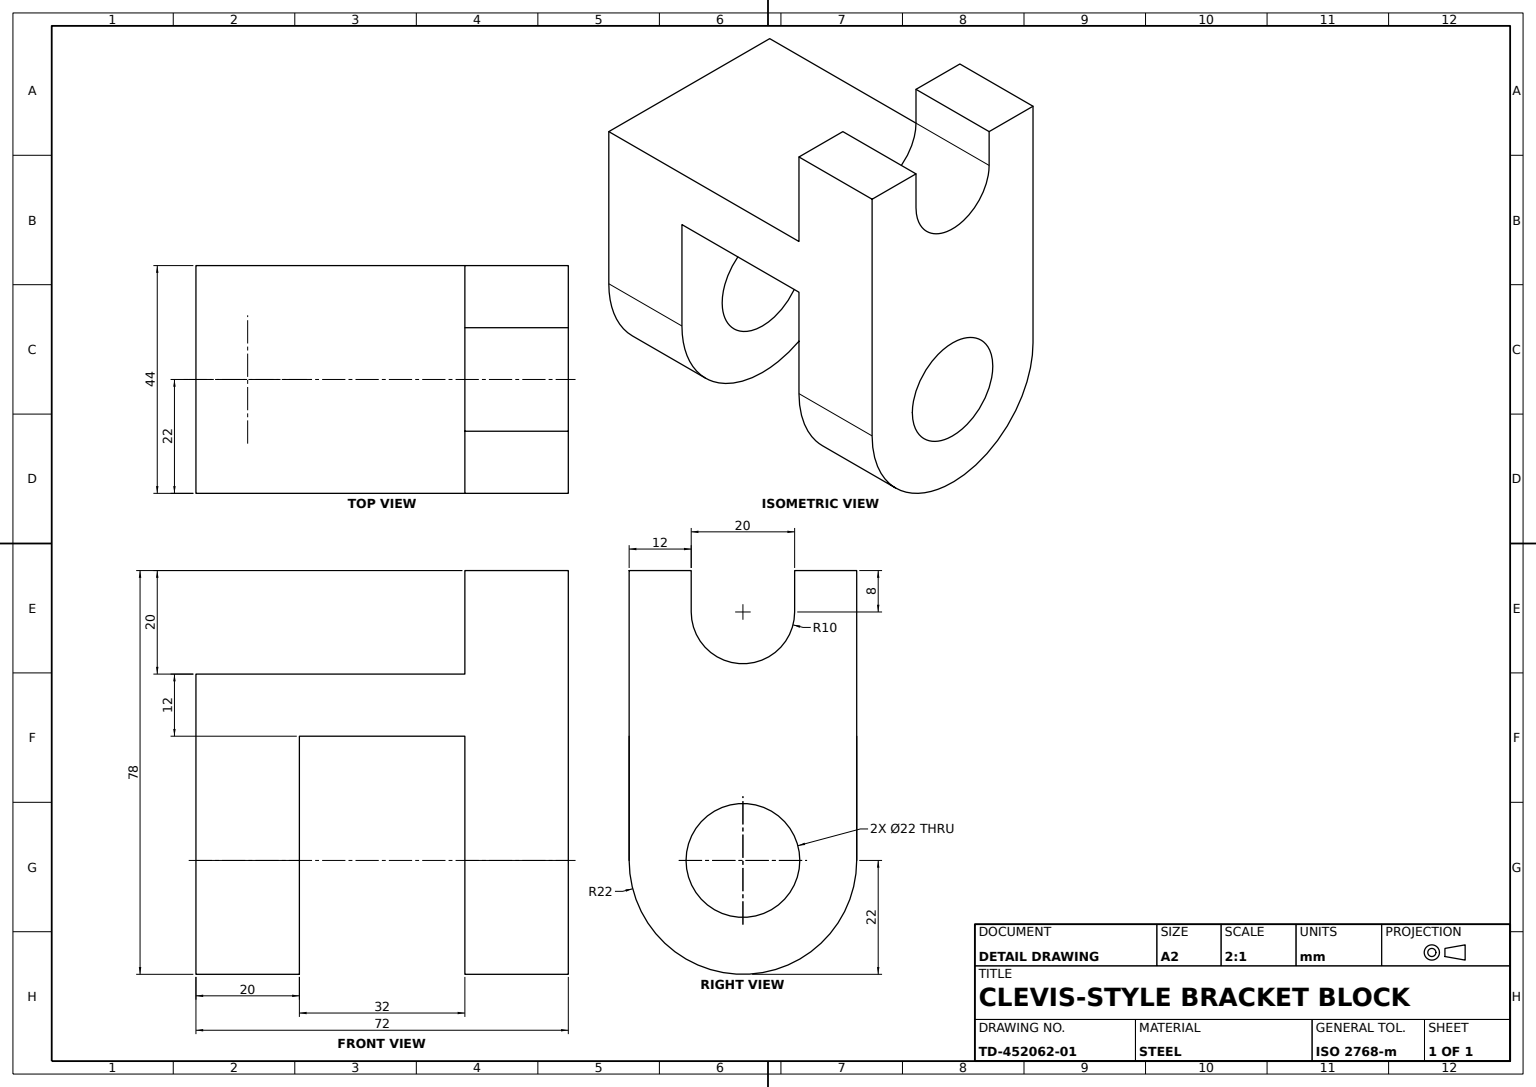
SolidWorks part; units mm, degrees
material "Plain Carbon Steel"
ref_plane "Front Plane" through (0, 0, 0) normal (0, 0, 1) x (1, 0, 0)
ref_plane "Top Plane" through (0, 0, 0) normal (0, 1, 0) x (1, 0, 0)
ref_plane "Right Plane" through (0, 0, 0) normal (1, 0, 0) x (0, 0, -1)
sketch "Base Profile Sketch" plane through (0, 0, 0) normal (0, 0, 1) x (1, 0, 0)
  line L0 (-36, 0) -> (36, 0)
  line L1 (36, 0) -> (36, 32)
  line L2 (36, 32) -> (16, 32)
  line L3 (16, 32) -> (16, 12)
  line L4 (16, 12) -> (-36, 12)
  line L5 (-36, 12) -> (-36, 0)
  point P4 (0, 0)
  dimension "D1" = 72
  dimension "D2" = 20
  dimension "D3" = 32
  dimension "D4" = 20
  dimension "D5" = 12
extrude "Base Block" add sketch "Base Profile Sketch" along normal mid plane 44
sketch "Lug Web Sketch" plane through (0, 0, 0) normal (0, -1, 0) x (1, 0, 0)
  line L0 (-36, 22) -> (-16, 22)
  line L1 (-36, 22) -> (36, 22) construction
  line L2 (-16, 22) -> (-16, -22)
  line L3 (-36, -22) -> (36, -22) construction
  line L4 (-16, -22) -> (-36, -22)
  line L5 (-36, -22) -> (-36, 22)
  line L6 (36, 22) -> (16, 22)
  line L7 (16, 22) -> (16, -22)
  line L8 (16, -22) -> (36, -22)
  line L9 (36, 22) -> (36, -22) construction
  line L10 (36, -22) -> (36, 22)
  dimension "D1" = 20
  dimension "D2" = 20
extrude "Lug Web" add sketch "Lug Web Sketch" along normal blind 24
sketch "Lug Boss 1 Sketch" plane through (-36, 0, 0) normal (-1, 0, 0) x (0, 0, 1)
  line L0 (22, -24) -> (-22, -24) construction
  circle A0 centre (0, -24) radius 22
  circle A1 centre (0, -24) radius 11
  dimension "D1" = 22
extrude "Lug Boss 1 R22" add sketch "Lug Boss 1 Sketch" against normal blind 20
sketch "Lug Hole 1 Sketch" plane through (-36, 0, 0) normal (-1, 0, 0) x (0, 0, 1)
  line L0 (11, -24) -> (-11, -24) construction
  circle A0 centre (0, -24) radius 11
  dimension "D1" = 22
extrude "Lug Hole 1" cut sketch "Lug Hole 1 Sketch" against normal blind 20
sketch "Lug Boss 2 Sketch" plane through (36, 0, 0) normal (1, 0, 0) x (0, 0, -1)
  line L0 (22, -24) -> (-22, -24) construction
  circle A0 centre (0, -24) radius 22
  circle A1 centre (0, -24) radius 11
  dimension "D1" = 22
  dimension "D2" = 44
extrude "Lug Boss 2 R22" add sketch "Lug Boss 2 Sketch" against normal blind 20
sketch "Lug Hole 2 Sketch" plane through (36, 0, 0) normal (1, 0, 0) x (0, 0, -1)
  line L0 (11, -24) -> (-11, -24) construction
  circle A0 centre (0, -24) radius 11
  dimension "D1" = 22
extrude "Lug Hole 2" cut sketch "Lug Hole 2 Sketch" against normal blind 20
sketch "Clevis Slot Sketch" plane through (16, 0, 0) normal (-1, 0, 0) x (0, 0, 1)
  line L0 (22, 32) -> (-22, 32) construction
  line L1 (-10, 24) -> (-10, 32)
  line L2 (10, 24) -> (10, 32)
  line L3 (-22, 32) -> (-22, 12) construction
  arc A0 (-10, 24) -> (10, 24) centre (0, 24) ccw
  dimension "D2" = 20
  dimension "D1" = 8
  dimension "D3" = 22
extrude "Clevis Slot" cut sketch "Clevis Slot Sketch" against normal blind 20 and the other way through all
